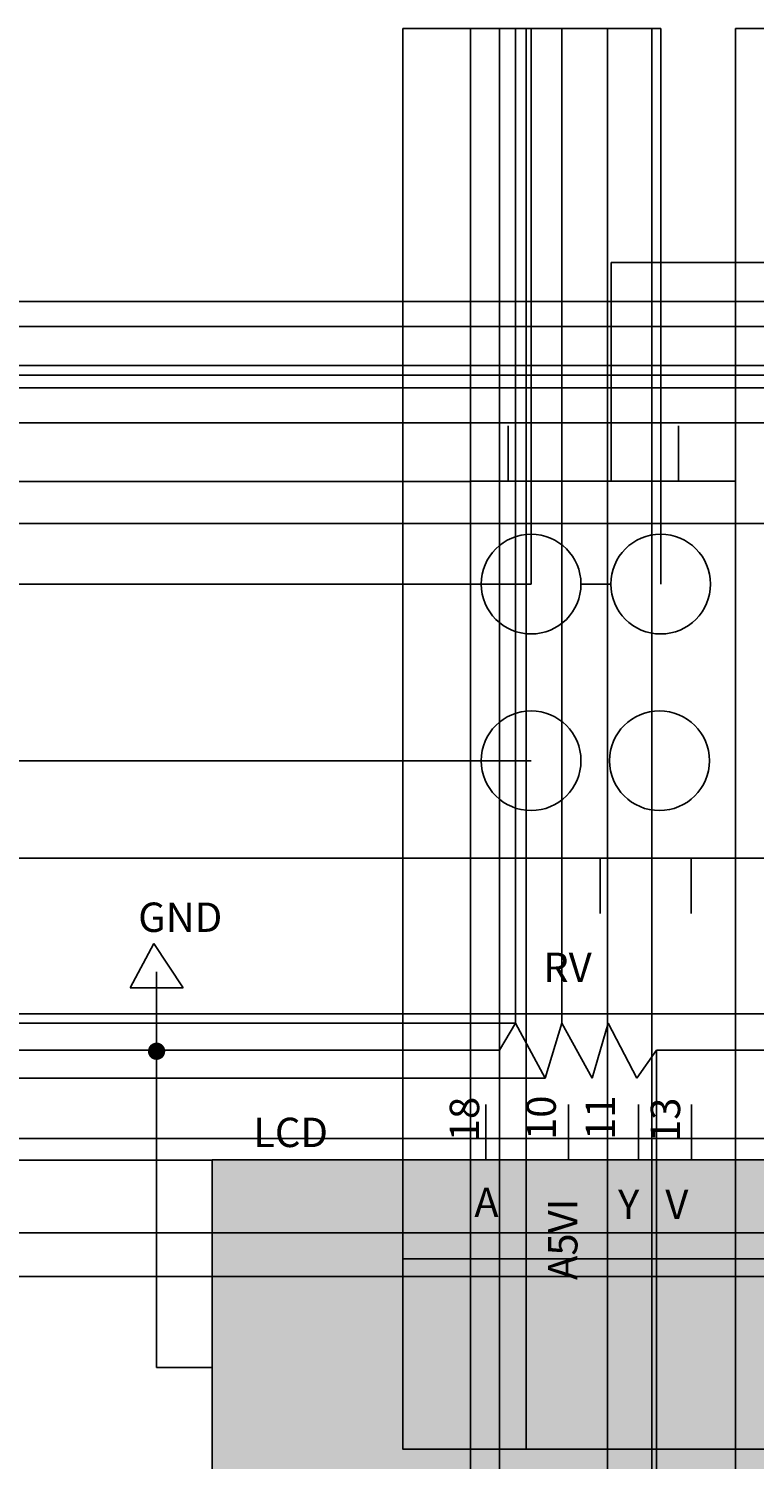
# Model space of a CAD drawing. Units: inches. Extents: x 35362 to 73946, y 43607 to 67532.
# Tile 130 of 134: x 46600 to 52056, y 56772 to 67532. Entities that reach past the tile are written whole.
import ezdxf

# ---------------------------------------------------------------- set-up
doc = ezdxf.new("R2010")
doc.units = ezdxf.units.IN
doc.header["$MEASUREMENT"] = 0
for name, color, linetype, lineweight in [('A-ANNO-DIMS', 2, 'Continuous', 18), ('E-ANNO-TEXT', 5, 'Continuous', 18), ('E-SYMB', 1, 'Continuous', 25), ('E-SYMB-PATT', 1, 'Continuous', 13), ('E-WIRE', 3, 'Continuous', 25)]:
    doc.layers.add(name, color=color, linetype=linetype, lineweight=lineweight)
doc.styles.get("Standard").update_dxf_attribs({"font": 'arial.ttf'})
doc.dimstyles.get("Standard").update_dxf_attribs({"dimtxt": 0.18, "dimasz": 0.18, "dimexe": 0.18, "dimexo": 0.0625, "dimgap": 0.09, "dimtad": 0, "dimtih": 1, "dimtoh": 1, "dimdec": 4, "dimzin": 0, "dimdsep": 46, "dimtxsty": 'Standard', "dimcen": 0.09, "dimadec": 0, "dimazin": 0, "dimtfac": 1, "dimtdec": 4, "dimtofl": 0, "dimtmove": 0, "dimatfit": 3, "dimfxl": 1, "dimtolj": 1, "dimtzin": 0, "dimarcsym": 0})

# ---------------------------------------------------------------- blocks, each defined once
blk = doc.blocks.new('*D12')
at = {"layer": 'A-ANNO-DIMS', "color": 0, "lineweight": -2, "transparency": 16777216}
for p, q in [((47979, 59023), (35362, 59023)), ((35362, 59023), (35362, 57526)), ((35362, 56029), (35362, 57526)), ((47979, 56029), (35362, 56029))]:
    blk.add_line(p, q, dxfattribs=at)
at = {"layer": 'A-ANNO-DIMS', "color": 0, "transparency": 16777216}
for points in [[(35362, 59023), (35362, 59023), (35362, 59023)], [(35362, 56029), (35362, 56029), (35362, 56029)]]:
    blk.add_solid(points, dxfattribs=at)
at = {"layer": 'Defpoints', "color": 0, "transparency": 16777216}
for p in [(47979, 59023), (35362, 56029), (47979, 56029)]:
    blk.add_point(p, dxfattribs=at)
at = {"layer": 'A-ANNO-DIMS', "color": 0, "transparency": 16777216, "insert": (35362, 57526), "char_height": 0.18, "attachment_point": 5}
blk.add_mtext('\\A1;2994.4', dxfattribs=at)
blk = doc.blocks.new('*D17')
at = {"layer": 'A-ANNO-DIMS', "color": 0, "lineweight": -2, "transparency": 16777216}
for p, q in [((49923, 61293), (49923, 43607)), ((51914, 61293), (51914, 43607)), ((49923, 43607), (50918, 43607)), ((51914, 43607), (50919, 43607))]:
    blk.add_line(p, q, dxfattribs=at)
at = {"layer": 'A-ANNO-DIMS', "color": 0, "transparency": 16777216}
for points in [[(49923, 43607), (49923, 43607), (49923, 43607)], [(51914, 43607), (51914, 43607), (51914, 43607)]]:
    blk.add_solid(points, dxfattribs=at)
at = {"layer": 'Defpoints', "color": 0, "transparency": 16777216}
for p in [(49923, 61293), (51914, 61293), (51914, 43607)]:
    blk.add_point(p, dxfattribs=at)
at = {"layer": 'A-ANNO-DIMS', "color": 0, "transparency": 16777216, "insert": (50919, 43607), "char_height": 0.18, "attachment_point": 5}
blk.add_mtext('\\A1;1990.6', dxfattribs=at)
blk = doc.blocks.new('*D18')
at = {"layer": 'A-ANNO-DIMS', "color": 0, "lineweight": -2, "transparency": 16777216}
for p, q in [((49923, 64127), (35362, 64127)), ((35362, 64127), (35362, 62711)), ((35362, 61293), (35362, 62710)), ((49923, 61293), (35362, 61293))]:
    blk.add_line(p, q, dxfattribs=at)
at = {"layer": 'A-ANNO-DIMS', "color": 0, "transparency": 16777216}
for points in [[(35362, 64127), (35362, 64127), (35362, 64127)], [(35362, 61293), (35362, 61293), (35362, 61293)]]:
    blk.add_solid(points, dxfattribs=at)
at = {"layer": 'Defpoints', "color": 0, "transparency": 16777216}
for p in [(49923, 64127), (35362, 61293), (49923, 61293)]:
    blk.add_point(p, dxfattribs=at)
at = {"layer": 'A-ANNO-DIMS', "color": 0, "transparency": 16777216, "insert": (35362, 62710), "char_height": 0.18, "attachment_point": 5}
blk.add_mtext('\\A1;2834', dxfattribs=at)
blk = doc.blocks.new('*D19')
at = {"layer": 'A-ANNO-DIMS', "color": 0, "lineweight": -2, "transparency": 16777216}
for p, q in [((50752, 63354), (50977, 63354)), ((51352, 63354), (51352, 63354)), ((51352, 63354), (51352, 63354))]:
    blk.add_line(p, q, dxfattribs=at)
at = {"layer": 'A-ANNO-DIMS', "color": 0, "transparency": 16777216}
blk.add_solid([(50977, 63354), (50977, 63354), (50977, 63354)], dxfattribs=at)
at = {"layer": 'Defpoints', "color": 0, "transparency": 16777216}
for p in [(50977, 63354), (51727, 63354)]:
    blk.add_point(p, dxfattribs=at)
at = {"layer": 'A-ANNO-DIMS', "color": 0, "transparency": 16777216, "insert": (50751, 63354), "char_height": 0.18, "attachment_point": 5}
blk.add_mtext('\\A1;8X ∅750.3', dxfattribs=at)
blk = doc.blocks.new('*D28')
at = {"layer": 'A-ANNO-DIMS', "color": 0, "lineweight": -2, "transparency": 16777216}
for p, q in [((49923, 61293), (35362, 61293)), ((35362, 61293), (35362, 60158)), ((35362, 59023), (35362, 60158)), ((47979, 59023), (35362, 59023))]:
    blk.add_line(p, q, dxfattribs=at)
at = {"layer": 'A-ANNO-DIMS', "color": 0, "transparency": 16777216}
for points in [[(35362, 61293), (35362, 61293), (35362, 61293)], [(35362, 59023), (35362, 59023), (35362, 59023)]]:
    blk.add_solid(points, dxfattribs=at)
at = {"layer": 'Defpoints', "color": 0, "transparency": 16777216}
for p in [(49923, 61293), (35362, 59023), (47979, 59023)]:
    blk.add_point(p, dxfattribs=at)
at = {"layer": 'A-ANNO-DIMS', "color": 0, "transparency": 16777216, "insert": (35362, 60158), "char_height": 0.18, "attachment_point": 5}
blk.add_mtext('\\A1;2270.0', dxfattribs=at)
blk = doc.blocks.new('*D29')
at = {"layer": 'A-ANNO-DIMS', "color": 0, "lineweight": -2, "transparency": 16777216}
for p, q in [((51914, 64128), (51914, 67532)), ((51914, 67532), (52215, 67532)), ((52518, 67532), (52216, 67532)), ((52518, 64829), (52518, 67532))]:
    blk.add_line(p, q, dxfattribs=at)
at = {"layer": 'A-ANNO-DIMS', "color": 0, "transparency": 16777216}
for points in [[(51914, 67532), (51914, 67531), (51914, 67532)], [(52518, 67532), (52518, 67531), (52518, 67532)]]:
    blk.add_solid(points, dxfattribs=at)
at = {"layer": 'Defpoints', "color": 0, "transparency": 16777216}
for p in [(52518, 67532), (52518, 64829), (51914, 64127)]:
    blk.add_point(p, dxfattribs=at)
at = {"layer": 'A-ANNO-DIMS', "color": 0, "transparency": 16777216, "insert": (52216, 67532), "char_height": 0.18, "attachment_point": 5}
blk.add_mtext('\\A1;603.9', dxfattribs=at)
blk = doc.blocks.new('*D34')
at = {"layer": 'A-ANNO-DIMS', "color": 0, "lineweight": -2, "transparency": 16777216}
for p, q in [((65336, 61293), (35362, 61293)), ((35362, 61293), (35362, 60239)), ((35362, 59185), (35362, 60239)), ((61241, 59185), (35362, 59185))]:
    blk.add_line(p, q, dxfattribs=at)
at = {"layer": 'A-ANNO-DIMS', "color": 0, "transparency": 16777216}
for points in [[(35362, 61293), (35362, 61293), (35362, 61293)], [(35362, 59185), (35362, 59185), (35362, 59185)]]:
    blk.add_solid(points, dxfattribs=at)
at = {"layer": 'Defpoints', "color": 0, "transparency": 16777216}
for p in [(65336, 61293), (35362, 59185), (61241, 59185)]:
    blk.add_point(p, dxfattribs=at)
at = {"layer": 'A-ANNO-DIMS', "color": 0, "transparency": 16777216, "insert": (35362, 60239), "char_height": 0.18, "attachment_point": 5}
blk.add_mtext('\\A1;2108.1', dxfattribs=at)
blk = doc.blocks.new('*D36')
at = {"layer": 'A-ANNO-DIMS', "color": 0, "lineweight": -2, "transparency": 16777216}
for p, q in [((68321, 60122), (35362, 60122)), ((35362, 60122), (35362, 57248)), ((35362, 54373), (35362, 57247)), ((68321, 54373), (35362, 54373))]:
    blk.add_line(p, q, dxfattribs=at)
at = {"layer": 'A-ANNO-DIMS', "color": 0, "transparency": 16777216}
for points in [[(35362, 60122), (35362, 60122), (35362, 60122)], [(35362, 54373), (35362, 54373), (35362, 54373)]]:
    blk.add_solid(points, dxfattribs=at)
at = {"layer": 'Defpoints', "color": 0, "transparency": 16777216}
for p in [(68321, 60122), (35362, 54373), (68321, 54373)]:
    blk.add_point(p, dxfattribs=at)
at = {"layer": 'A-ANNO-DIMS', "color": 0, "transparency": 16777216, "insert": (35362, 57248), "char_height": 0.18, "attachment_point": 5}
blk.add_mtext('\\A1;5749.4', dxfattribs=at)
blk = doc.blocks.new('*D45')
at = {"layer": 'A-ANNO-DIMS', "color": 0, "lineweight": -2, "transparency": 16777216}
for p, q in [((52518, 65479), (35362, 65479)), ((35362, 65479), (35362, 65154)), ((35362, 64829), (35362, 65154)), ((52518, 64829), (35362, 64829))]:
    blk.add_line(p, q, dxfattribs=at)
at = {"layer": 'A-ANNO-DIMS', "color": 0, "transparency": 16777216}
for points in [[(35362, 65479), (35362, 65479), (35362, 65479)], [(35362, 64829), (35362, 64829), (35362, 64829)]]:
    blk.add_solid(points, dxfattribs=at)
at = {"layer": 'Defpoints', "color": 0, "transparency": 16777216}
for p in [(52518, 65479), (35362, 64829), (52518, 64829)]:
    blk.add_point(p, dxfattribs=at)
at = {"layer": 'A-ANNO-DIMS', "color": 0, "transparency": 16777216, "insert": (35362, 65154), "char_height": 0.18, "attachment_point": 5}
blk.add_mtext('\\A1;650.3', dxfattribs=at)
blk = doc.blocks.new('*D46')
at = {"layer": 'A-ANNO-DIMS', "color": 0, "lineweight": -2, "transparency": 16777216}
for p, q in [((49414, 58280), (49414, 67532)), ((49414, 67532), (49876, 67532)), ((50339, 67532), (49877, 67532)), ((50340, 58280), (50340, 67532))]:
    blk.add_line(p, q, dxfattribs=at)
at = {"layer": 'A-ANNO-DIMS', "color": 0, "transparency": 16777216}
for points in [[(49414, 67532), (49414, 67531), (49414, 67532)], [(50339, 67532), (50339, 67531), (50340, 67532)]]:
    blk.add_solid(points, dxfattribs=at)
at = {"layer": 'Defpoints', "color": 0, "transparency": 16777216}
for p in [(50340, 67532), (49414, 58280), (50340, 58280)]:
    blk.add_point(p, dxfattribs=at)
at = {"layer": 'A-ANNO-DIMS', "color": 0, "transparency": 16777216, "insert": (49877, 67532), "char_height": 0.18, "attachment_point": 5}
blk.add_mtext('\\A1;925.3', dxfattribs=at)
blk = doc.blocks.new('*D47')
at = {"layer": 'A-ANNO-DIMS', "color": 0, "lineweight": -2, "transparency": 16777216}
for p, q in [((50340, 58280), (73946, 58280)), ((73946, 58280), (73946, 57564)), ((73946, 56848), (73946, 57564)), ((50340, 56848), (73946, 56848))]:
    blk.add_line(p, q, dxfattribs=at)
at = {"layer": 'A-ANNO-DIMS', "color": 0, "transparency": 16777216}
for points in [[(73946, 58280), (73946, 58280), (73946, 58280)], [(73946, 56848), (73946, 56848), (73946, 56848)]]:
    blk.add_solid(points, dxfattribs=at)
at = {"layer": 'Defpoints', "color": 0, "transparency": 16777216}
for p in [(50340, 58280), (50340, 56848), (73946, 56848)]:
    blk.add_point(p, dxfattribs=at)
at = {"layer": 'A-ANNO-DIMS', "color": 0, "transparency": 16777216, "insert": (73946, 57564), "char_height": 0.18, "attachment_point": 5}
blk.add_mtext('\\A1;1432.0', dxfattribs=at)
blk = doc.blocks.new('*D48')
at = {"layer": 'A-ANNO-DIMS', "color": 0, "lineweight": -2, "transparency": 16777216}
for p, q in [((56457, 58475), (35362, 58475)), ((35362, 58475), (35362, 58311)), ((35362, 58147), (35362, 58311)), ((56457, 58147), (35362, 58147))]:
    blk.add_line(p, q, dxfattribs=at)
at = {"layer": 'A-ANNO-DIMS', "color": 0, "transparency": 16777216}
for points in [[(35362, 58475), (35362, 58475), (35362, 58475)], [(35362, 58147), (35362, 58147), (35362, 58147)]]:
    blk.add_solid(points, dxfattribs=at)
at = {"layer": 'Defpoints', "color": 0, "transparency": 16777216}
for p in [(56457, 58475), (35362, 58147), (56457, 58147)]:
    blk.add_point(p, dxfattribs=at)
at = {"layer": 'A-ANNO-DIMS', "color": 0, "transparency": 16777216, "insert": (35362, 58311), "char_height": 0.18, "attachment_point": 5}
blk.add_mtext('\\A1;327.9', dxfattribs=at)
blk = doc.blocks.new('*D59')
at = {"layer": 'A-ANNO-DIMS', "color": 0, "lineweight": -2, "transparency": 16777216}
for p, q in [((50752, 63354), (50977, 63354)), ((51352, 63354), (51352, 63354)), ((51352, 63354), (51352, 63354))]:
    blk.add_line(p, q, dxfattribs=at)
at = {"layer": 'A-ANNO-DIMS', "color": 0, "transparency": 16777216}
blk.add_solid([(50977, 63354), (50977, 63354), (50977, 63354)], dxfattribs=at)
at = {"layer": 'Defpoints', "color": 0, "transparency": 16777216}
for p in [(50977, 63354), (51727, 63354)]:
    blk.add_point(p, dxfattribs=at)
at = {"layer": 'A-ANNO-DIMS', "color": 0, "transparency": 16777216, "insert": (50751, 63354), "char_height": 0.18, "attachment_point": 5}
blk.add_mtext('\\A1;8X ∅750.3', dxfattribs=at)
blk = doc.blocks.new('*D73')
at = {"layer": 'A-ANNO-DIMS', "color": 0, "lineweight": -2, "transparency": 16777216}
for p, q in [((59469, 64568), (35362, 64568)), ((35362, 64568), (35362, 64190)), ((35362, 63812), (35362, 64189)), ((59469, 63811), (35362, 63811))]:
    blk.add_line(p, q, dxfattribs=at)
at = {"layer": 'A-ANNO-DIMS', "color": 0, "transparency": 16777216}
for points in [[(35362, 64568), (35362, 64568), (35362, 64568)], [(35362, 63812), (35362, 63812), (35362, 63811)]]:
    blk.add_solid(points, dxfattribs=at)
at = {"layer": 'Defpoints', "color": 0, "transparency": 16777216}
for p in [(35362, 64568), (59469, 64568), (59469, 63811)]:
    blk.add_point(p, dxfattribs=at)
at = {"layer": 'A-ANNO-DIMS', "color": 0, "transparency": 16777216, "insert": (35362, 64190), "char_height": 0.18, "attachment_point": 5}
blk.add_mtext('\\A1;756.6', dxfattribs=at)
blk = doc.blocks.new('*D85')
at = {"layer": 'A-ANNO-DIMS', "color": 0, "lineweight": -2, "transparency": 16777216}
for p, q in [((50953, 49098), (50953, 67532)), ((50953, 67532), (51119, 67532)), ((51285, 67532), (51120, 67532)), ((51286, 49320), (51286, 67532))]:
    blk.add_line(p, q, dxfattribs=at)
at = {"layer": 'A-ANNO-DIMS', "color": 0, "transparency": 16777216}
for points in [[(50953, 67532), (50953, 67531), (50953, 67532)], [(51285, 67532), (51285, 67531), (51286, 67532)]]:
    blk.add_solid(points, dxfattribs=at)
at = {"layer": 'Defpoints', "color": 0, "transparency": 16777216}
for p in [(51286, 67532), (51286, 49320), (50953, 49098)]:
    blk.add_point(p, dxfattribs=at)
at = {"layer": 'A-ANNO-DIMS', "color": 0, "transparency": 16777216, "insert": (51119, 67532), "char_height": 0.18, "attachment_point": 5}
blk.add_mtext('\\A1;332.9', dxfattribs=at)
blk = doc.blocks.new('*D92')
at = {"layer": 'A-ANNO-DIMS', "color": 0, "lineweight": -2, "transparency": 16777216}
for p, q in [((50378, 63354), (50378, 67532)), ((50378, 67532), (50864, 67532)), ((51352, 67532), (50865, 67532)), ((51352, 63354), (51352, 67532))]:
    blk.add_line(p, q, dxfattribs=at)
at = {"layer": 'A-ANNO-DIMS', "color": 0, "transparency": 16777216}
for points in [[(50378, 67532), (50378, 67531), (50378, 67532)], [(51352, 67532), (51352, 67531), (51352, 67532)]]:
    blk.add_solid(points, dxfattribs=at)
at = {"layer": 'Defpoints', "color": 0, "transparency": 16777216}
for p in [(51352, 67532), (50378, 63354), (51352, 63354)]:
    blk.add_point(p, dxfattribs=at)
at = {"layer": 'A-ANNO-DIMS', "color": 0, "transparency": 16777216, "insert": (50865, 67532), "char_height": 0.18, "attachment_point": 5}
blk.add_mtext('\\A1;974.2', dxfattribs=at)
blk = doc.blocks.new('*D93')
at = {"layer": 'A-ANNO-DIMS', "color": 0, "lineweight": -2, "transparency": 16777216}
for p, q in [((50378, 63354), (35362, 63354)), ((35362, 63354), (35362, 62690)), ((35362, 62026), (35362, 62690)), ((50378, 62026), (35362, 62026))]:
    blk.add_line(p, q, dxfattribs=at)
at = {"layer": 'A-ANNO-DIMS', "color": 0, "transparency": 16777216}
for points in [[(35362, 63354), (35362, 63354), (35362, 63354)], [(35362, 62026), (35362, 62026), (35362, 62026)]]:
    blk.add_solid(points, dxfattribs=at)
at = {"layer": 'Defpoints', "color": 0, "transparency": 16777216}
for p in [(50378, 63354), (35362, 62026), (50378, 62026)]:
    blk.add_point(p, dxfattribs=at)
at = {"layer": 'A-ANNO-DIMS', "color": 0, "transparency": 16777216, "insert": (35362, 62690), "char_height": 0.18, "attachment_point": 5}
blk.add_mtext('\\A1;1328.2', dxfattribs=at)
blk = doc.blocks.new('*D94')
at = {"layer": 'A-ANNO-DIMS', "color": 0, "lineweight": -2, "transparency": 16777216}
for p, q in [((49923, 64128), (49923, 67532)), ((49923, 67532), (50150, 67532)), ((50378, 67532), (50151, 67532)), ((50378, 63354), (50378, 67532))]:
    blk.add_line(p, q, dxfattribs=at)
at = {"layer": 'A-ANNO-DIMS', "color": 0, "transparency": 16777216}
for points in [[(49923, 67532), (49923, 67531), (49923, 67532)], [(50378, 67532), (50378, 67531), (50378, 67532)]]:
    blk.add_solid(points, dxfattribs=at)
at = {"layer": 'Defpoints', "color": 0, "transparency": 16777216}
for p in [(50378, 67532), (49923, 64127), (50378, 63354)]:
    blk.add_point(p, dxfattribs=at)
at = {"layer": 'A-ANNO-DIMS', "color": 0, "transparency": 16777216, "insert": (50151, 67532), "char_height": 0.18, "attachment_point": 5}
blk.add_mtext('\\A1;454.45', dxfattribs=at)
blk = doc.blocks.new('*D95')
at = {"layer": 'A-ANNO-DIMS', "color": 0, "lineweight": -2, "transparency": 16777216}
for p, q in [((49923, 64127), (35362, 64127)), ((35362, 64127), (35362, 63741)), ((35362, 63354), (35362, 63741)), ((50378, 63354), (35362, 63354))]:
    blk.add_line(p, q, dxfattribs=at)
at = {"layer": 'A-ANNO-DIMS', "color": 0, "transparency": 16777216}
for points in [[(35362, 64127), (35362, 64127), (35362, 64127)], [(35362, 63354), (35362, 63354), (35362, 63354)]]:
    blk.add_solid(points, dxfattribs=at)
at = {"layer": 'Defpoints', "color": 0, "transparency": 16777216}
for p in [(49923, 64127), (35362, 63354), (50378, 63354)]:
    blk.add_point(p, dxfattribs=at)
at = {"layer": 'A-ANNO-DIMS', "color": 0, "transparency": 16777216, "insert": (35362, 63741), "char_height": 0.18, "attachment_point": 5}
blk.add_mtext('\\A1;773.3', dxfattribs=at)
blk = doc.blocks.new('*D98')
at = {"layer": 'A-ANNO-DIMS', "color": 0, "lineweight": -2, "transparency": 16777216}
for p, q in [((53367, 64998), (35362, 64998)), ((35362, 64998), (35362, 64913)), ((35362, 64829), (35362, 64913)), ((52518, 64829), (35362, 64829))]:
    blk.add_line(p, q, dxfattribs=at)
at = {"layer": 'A-ANNO-DIMS', "color": 0, "transparency": 16777216}
for points in [[(35362, 64998), (35362, 64998), (35362, 64998)], [(35362, 64829), (35362, 64829), (35362, 64829)]]:
    blk.add_solid(points, dxfattribs=at)
at = {"layer": 'Defpoints', "color": 0, "transparency": 16777216}
for p in [(53367, 64998), (35362, 64829), (52518, 64829)]:
    blk.add_point(p, dxfattribs=at)
at = {"layer": 'A-ANNO-DIMS', "color": 0, "transparency": 16777216, "insert": (35362, 64913), "char_height": 0.18, "attachment_point": 5}
blk.add_mtext('\\A1;169.13', dxfattribs=at)
blk = doc.blocks.new('*D101')
at = {"layer": 'A-ANNO-DIMS', "color": 0, "lineweight": -2, "transparency": 16777216}
for p, q in [((52897, 65292), (35362, 65292)), ((35362, 65291), (35362, 65109)), ((35362, 64926), (35362, 65109)), ((53151, 64926), (35362, 64926))]:
    blk.add_line(p, q, dxfattribs=at)
at = {"layer": 'A-ANNO-DIMS', "color": 0, "transparency": 16777216}
for points in [[(35362, 65291), (35362, 65291), (35362, 65292)], [(35362, 64926), (35362, 64926), (35362, 64926)]]:
    blk.add_solid(points, dxfattribs=at)
at = {"layer": 'Defpoints', "color": 0, "transparency": 16777216}
for p in [(52897, 65292), (35362, 64926), (53151, 64926)]:
    blk.add_point(p, dxfattribs=at)
at = {"layer": 'A-ANNO-DIMS', "color": 0, "transparency": 16777216, "insert": (35362, 65109), "char_height": 0.18, "attachment_point": 5}
blk.add_mtext('\\A1;365.45', dxfattribs=at)
blk = doc.blocks.new('*D107')
at = {"layer": 'A-ANNO-DIMS', "color": 0, "lineweight": -2, "transparency": 16777216}
for p, q in [((50140, 59850), (50140, 43607)), ((51321, 59850), (51321, 43607)), ((50140, 43607), (50730, 43607)), ((51321, 43607), (50731, 43607))]:
    blk.add_line(p, q, dxfattribs=at)
at = {"layer": 'A-ANNO-DIMS', "color": 0, "transparency": 16777216}
for points in [[(50140, 43607), (50140, 43607), (50140, 43607)], [(51321, 43607), (51321, 43607), (51321, 43607)]]:
    blk.add_solid(points, dxfattribs=at)
at = {"layer": 'Defpoints', "color": 0, "transparency": 16777216}
for p in [(50140, 59850), (51321, 59850), (51321, 43607)]:
    blk.add_point(p, dxfattribs=at)
at = {"layer": 'A-ANNO-DIMS', "color": 0, "transparency": 16777216, "insert": (50730, 43607), "char_height": 0.18, "attachment_point": 5}
blk.add_mtext('\\A1;1181.3', dxfattribs=at)
blk = doc.blocks.new('*D108')
at = {"layer": 'A-ANNO-DIMS', "color": 0, "lineweight": -2, "transparency": 16777216}
for p, q in [((50260, 60052), (35362, 60052)), ((35362, 60051), (35362, 59845)), ((35362, 59638), (35362, 59845)), ((50483, 59638), (35362, 59638))]:
    blk.add_line(p, q, dxfattribs=at)
at = {"layer": 'A-ANNO-DIMS', "color": 0, "transparency": 16777216}
for points in [[(35362, 60051), (35362, 60051), (35362, 60052)], [(35362, 59638), (35362, 59638), (35362, 59638)]]:
    blk.add_solid(points, dxfattribs=at)
at = {"layer": 'Defpoints', "color": 0, "transparency": 16777216}
for p in [(50260, 60052), (35362, 59638), (50483, 59638)]:
    blk.add_point(p, dxfattribs=at)
at = {"layer": 'A-ANNO-DIMS', "color": 0, "transparency": 16777216, "insert": (35362, 59845), "char_height": 0.18, "attachment_point": 5}
blk.add_mtext('\\A1;413.5', dxfattribs=at)
blk = doc.blocks.new('*D109')
at = {"layer": 'A-ANNO-DIMS', "color": 0, "lineweight": -2, "transparency": 16777216}
for p, q in [((50260, 60052), (50260, 67532)), ((50260, 67532), (50434, 67532)), ((50610, 67532), (50435, 67532)), ((50610, 60052), (50610, 67532))]:
    blk.add_line(p, q, dxfattribs=at)
at = {"layer": 'A-ANNO-DIMS', "color": 0, "transparency": 16777216}
for points in [[(50260, 67532), (50260, 67531), (50260, 67532)], [(50610, 67532), (50610, 67531), (50610, 67532)]]:
    blk.add_solid(points, dxfattribs=at)
at = {"layer": 'Defpoints', "color": 0, "transparency": 16777216}
for p in [(50610, 67532), (50260, 60052), (50610, 60052)]:
    blk.add_point(p, dxfattribs=at)
at = {"layer": 'A-ANNO-DIMS', "color": 0, "transparency": 16777216, "insert": (50435, 67532), "char_height": 0.18, "attachment_point": 5}
blk.add_mtext('\\A1;350.2', dxfattribs=at)
blk = doc.blocks.new('*D110')
at = {"layer": 'A-ANNO-DIMS', "color": 0, "lineweight": -2, "transparency": 16777216}
for p, q in [((49923, 61293), (35362, 61293)), ((35362, 61293), (35362, 60572)), ((35362, 59850), (35362, 60571)), ((50140, 59850), (35362, 59850))]:
    blk.add_line(p, q, dxfattribs=at)
at = {"layer": 'A-ANNO-DIMS', "color": 0, "transparency": 16777216}
for points in [[(35362, 61293), (35362, 61293), (35362, 61293)], [(35362, 59850), (35362, 59850), (35362, 59850)]]:
    blk.add_solid(points, dxfattribs=at)
at = {"layer": 'Defpoints', "color": 0, "transparency": 16777216}
for p in [(49923, 61293), (35362, 59850), (50140, 59850)]:
    blk.add_point(p, dxfattribs=at)
at = {"layer": 'A-ANNO-DIMS', "color": 0, "transparency": 16777216, "insert": (35362, 60572), "char_height": 0.18, "attachment_point": 5}
blk.add_mtext('\\A1;1443.2', dxfattribs=at)
blk = doc.blocks.new('*D111')
at = {"layer": 'A-ANNO-DIMS', "color": 0, "lineweight": -2, "transparency": 16777216}
for p, q in [((49923, 61293), (49923, 67532)), ((49923, 67532), (50031, 67532)), ((50139, 67532), (50032, 67532)), ((50140, 59850), (50140, 67532))]:
    blk.add_line(p, q, dxfattribs=at)
at = {"layer": 'A-ANNO-DIMS', "color": 0, "transparency": 16777216}
for points in [[(49923, 67532), (49923, 67531), (49923, 67532)], [(50139, 67532), (50139, 67531), (50140, 67532)]]:
    blk.add_solid(points, dxfattribs=at)
at = {"layer": 'Defpoints', "color": 0, "transparency": 16777216}
for p in [(50140, 67532), (49923, 61293), (50140, 59850)]:
    blk.add_point(p, dxfattribs=at)
at = {"layer": 'A-ANNO-DIMS', "color": 0, "transparency": 16777216, "insert": (50031, 67532), "char_height": 0.18, "attachment_point": 5}
blk.add_mtext('\\A1;216.26', dxfattribs=at)
blk = doc.blocks.new('*D118')
at = {"layer": 'A-ANNO-DIMS', "color": 0, "lineweight": -2, "transparency": 16777216}
for p, q in [((50378, 63354), (50378, 63354)), ((50378, 63354), (50378, 63354)), ((50978, 63354), (50753, 63354))]:
    blk.add_line(p, q, dxfattribs=at)
at = {"layer": 'A-ANNO-DIMS', "color": 0, "transparency": 16777216}
blk.add_solid([(50753, 63354), (50753, 63354), (50753, 63354)], dxfattribs=at)
at = {"layer": 'Defpoints', "color": 0, "transparency": 16777216}
for p in [(50003, 63354), (50753, 63354)]:
    blk.add_point(p, dxfattribs=at)
at = {"layer": 'A-ANNO-DIMS', "color": 0, "transparency": 16777216, "insert": (50979, 63354), "char_height": 0.18, "attachment_point": 5}
blk.add_mtext('\\A1;8X ∅750.3', dxfattribs=at)

msp = doc.modelspace()

# ---------------------------------------------------------------- hatches: boundary and pattern name
at = {"layer": 'E-SYMB-PATT'}
h = msp.add_hatch(color=256, dxfattribs=at)
h.dxf.hatch_style = 1
h.paths.add_polyline_path([(47561.92, 59906.061, 0.414213562), (47496.715, 59840.856, 0.414213562), (47561.92, 59775.651)])
h.paths.add_polyline_path([(47561.92, 59906.061), (47561.92, 59775.651, 0.414213562), (47627.125, 59840.856, 0.414213562)])
h = msp.add_hatch(color=256, dxfattribs=at)
h.dxf.hatch_style = 1
h.paths.add_polyline_path([(53109.76, 56028.836), (53109.76, 59023.276), (47978.665, 59023.276), (47978.665, 56028.836)])

# ---------------------------------------------------------------- linework, layer by layer
at = {"layer": 'E-SYMB'}
for p, q in [((50978.723, 65771.512), (52897.48, 65771.512)), ((50204.468, 64543.754), (50204.468, 64127.442)), ((51485.882, 64543.754), (51485.882, 64127.442)), ((50340.575, 61293.286), (50340.575, 60876.974)), ((50898.169, 61293.286), (50898.169, 60876.974)), ((51581.922, 61293.286), (51581.922, 60876.974)), ((47540.642, 60650.854), (47362.353, 60317.921)), ((47762.353, 60317.921), (47540.642, 60650.854)), ((47562.353, 60317.921), (47362.353, 60317.921)), ((47562.353, 59850.077), (47562.353, 60317.921)), ((47562.353, 60317.921), (47762.353, 60317.921)), ((50139.563, 59850.077), (50259.724, 60051.661)), ((50259.724, 60051.661), (50483.095, 59638.132)), ((50483.095, 59638.132), (50609.914, 60051.661)), ((50609.914, 60051.661), (50836.506, 59638.132)), ((50836.506, 59638.132), (50956.669, 60051.661)), ((50956.669, 60051.661), (51172.962, 59638.132)), ((49903.185, 59850.077), (50139.563, 59850.077)), ((51172.962, 59638.132), (51320.813, 59850.077)), ((51320.813, 59850.077), (51612.51, 59850.077)), ((50038.496, 59439.589), (50038.496, 59023.276)), ((50658.098, 59439.589), (50658.098, 59023.276)), ((51185.224, 59439.589), (51185.224, 59023.276)), ((51582.878, 59439.589), (51582.878, 59023.276)), ((47978.665, 57463.179), (47562.353, 57463.179))]:
    msp.add_line(p, q, dxfattribs=at)
for points in [[(49923.307, 64127.442), (51913.931, 64127.442), (51913.931, 61293.286), (49923.307, 61293.286)], [(47978.665, 59023.276), (53109.76, 59023.276), (53109.76, 56028.836), (47978.665, 56028.836)], [(49414.26, 58279.988), (50339.524, 58279.988), (50339.524, 56847.99), (49414.26, 56847.99)]]:
    msp.add_lwpolyline(points, close=True, dxfattribs=at)
for centre in [(50377.76, 63354.176), (51351.915, 63354.176), (50377.76, 62026.025), (51342.885, 62026.025)]:
    msp.add_circle(centre, 375.127, dxfattribs=at)
at = {"layer": 'E-WIRE'}
for p, q in [((50978.723, 65771.512), (50978.723, 64127.442)), ((47562.353, 60439.178), (47562.353, 57463.179)), ((47562.353, 59850.077), (49903.185, 59850.077)), ((51612.51, 59850.077), (53526.072, 59850.077))]:
    msp.add_line(p, q, dxfattribs=at)

# ---------------------------------------------------------------- texts
at = {"layer": 'E-ANNO-TEXT'}
for s, p in [('GND', (47423.417, 60738.292)), ('RV', (50468.698, 60362.066)), ('LCD', (48287.73, 59120.329)), ('A', (49950.554, 58593.417)), ('Y', (51031.177, 58579.088)), ('V', (51386.782, 58579.088))]:
    msp.add_text(s, height=220.866, dxfattribs=at).set_placement(p)
for s, p in [('18', (49986.996, 59163.807)), ('10', (50563.845, 59173.51)), ('11', (51008.62, 59173.51)), ('13', (51498.496, 59158.048)), ('A5VI', (50726.347, 58120.572))]:
    msp.add_text(s, height=220.866, rotation=90, dxfattribs=at).set_placement(p)

# ---------------------------------------------------------------- dimensions: what is measured, and where the dimension line sits
at = {"layer": 'A-ANNO-DIMS'}
for base, p1, p2, override, picture, middle in [((50339.524, 67531.512), (49414.26, 58279.988), (50339.524, 58279.988), {"dimdec": 1, "dimlfac": 1, "dimrnd": 0, "dimzin": 0, "dimdsep": 46, "dimlunit": 2}, '*D46', (49876.892, 67531.512)), ((50377.76, 67531.512), (49923.307, 64127.442), (50377.76, 63354.176), {"dimdec": 2, "dimlfac": 1, "dimrnd": 0, "dimzin": 0, "dimdsep": 46, "dimlunit": 2}, '*D94', (50150.533, 67531.512)), ((50139.563, 67531.512), (49923.307, 61293.286), (50139.563, 59850.077), {"dimdec": 2, "dimlfac": 1, "dimrnd": 0, "dimzin": 0, "dimdsep": 46, "dimlunit": 2}, '*D111', (50031.435, 67531.512)), ((50609.914, 67531.512), (50259.724, 60051.661), (50609.914, 60051.661), {"dimdec": 1, "dimlfac": 1, "dimrnd": 0, "dimzin": 0, "dimdsep": 46, "dimlunit": 2}, '*D109', (50434.819, 67531.512)), ((51351.915, 67531.512), (50377.76, 63354.176), (51351.915, 63354.176), {"dimdec": 1, "dimlfac": 1, "dimrnd": 0, "dimzin": 0, "dimdsep": 46, "dimlunit": 2}, '*D92', (50864.837, 67531.512)), ((51285.595, 67531.512), (50952.662, 49098.368), (51285.595, 49320.079), {"dimdec": 1, "dimlfac": 1, "dimrnd": 0, "dimzin": 0, "dimdsep": 46, "dimlunit": 2}, '*D85', (51119.128, 67531.512)), ((52517.798, 67531.512), (51913.931, 64127.442), (52517.798, 64828.556), {"dimdec": 1, "dimlfac": 1, "dimrnd": 0, "dimzin": 0, "dimdsep": 46, "dimlunit": 2}, '*D29', (52215.864, 67531.512)), ((51913.931, 43606.859), (49923.307, 61293.286), (51913.931, 61293.286), {"dimdec": 1, "dimlfac": 1, "dimrnd": 0, "dimzin": 0, "dimdsep": 46, "dimlunit": 2}, '*D17', (50918.619, 43606.859)), ((51320.8133, 43606.859), (50139.5627, 59850.0769), (51320.8133, 59850.0769), {"dimdec": 1, "dimlfac": 1, "dimrnd": 0, "dimzin": 0, "dimdsep": 46, "dimlunit": 2}, '*D107', (50730.188, 43606.859))]:
    dim = msp.add_linear_dim(base=base, p1=p1, p2=p2, dimstyle='Standard', override=override, dxfattribs=at)
    dim.commit()
    dim.dimension.update_dxf_attribs({"geometry": picture, "text_midpoint": middle})
for base, p1, p2, override, picture, middle in [((35361.949, 64828.556), (52517.798, 65478.87), (52517.798, 64828.556), {"dimdec": 1, "dimlfac": 1, "dimrnd": 0, "dimzin": 0, "dimdsep": 46, "dimlunit": 2}, '*D45', (35361.949, 65153.713)), ((35361.949, 64926.138), (52897.48, 65291.589), (53150.662, 64926.138), {"dimdec": 2, "dimlfac": 1, "dimrnd": 0, "dimzin": 0, "dimdsep": 46, "dimlunit": 2}, '*D101', (35361.949, 65108.863)), ((35361.949, 64828.556), (53366.766, 64997.683), (52517.798, 64828.556), {"dimdec": 2, "dimlfac": 1, "dimrnd": 0, "dimzin": 0, "dimdsep": 46, "dimlunit": 2}, '*D98', (35361.949, 64913.119)), ((35361.949, 64567.972), (59468.796, 63811.354), (59468.796, 64567.972), {"dimdec": 1, "dimlfac": 1, "dimrnd": 0, "dimzin": 0, "dimdsep": 46, "dimlunit": 2}, '*D73', (35361.949, 64189.663)), ((35361.949, 63354.176), (49923.307, 64127.442), (50377.76, 63354.176), {"dimdec": 1, "dimlfac": 1, "dimrnd": 0, "dimzin": 0, "dimdsep": 46, "dimlunit": 2}, '*D95', (35361.949, 63740.809)), ((35361.949, 61293.286), (49923.307, 64127.442), (49923.307, 61293.286), {"dimdec": 0, "dimlfac": 1, "dimrnd": 0, "dimzin": 0, "dimdsep": 46, "dimlunit": 2}, '*D18', (35361.949, 62710.364)), ((35361.949, 62026.025), (50377.76, 63354.176), (50377.76, 62026.025), {"dimdec": 1, "dimlfac": 1, "dimrnd": 0, "dimzin": 0, "dimdsep": 46, "dimlunit": 2}, '*D93', (35361.949, 62690.1)), ((35361.949, 59023.276), (49923.307, 61293.286), (47978.665, 59023.276), {"dimdec": 1, "dimlfac": 1, "dimrnd": 0, "dimzin": 0, "dimdsep": 46, "dimlunit": 2}, '*D28', (35361.949, 60158.281)), ((35361.949, 59185.144), (65336.016, 61293.286), (61240.907, 59185.144), {"dimdec": 1, "dimlfac": 1, "dimrnd": 0, "dimzin": 0, "dimdsep": 46, "dimlunit": 2}, '*D34', (35361.949, 60239.215)), ((35361.949, 59850.077), (49923.307, 61293.286), (50139.563, 59850.077), {"dimdec": 1, "dimlfac": 1, "dimrnd": 0, "dimzin": 0, "dimdsep": 46, "dimlunit": 2}, '*D110', (35361.949, 60571.681)), ((35361.949, 54372.948), (68320.871, 60122.346), (68320.871, 54372.948), {"dimdec": 1, "dimlfac": 1, "dimrnd": 0, "dimzin": 0, "dimdsep": 46, "dimlunit": 2}, '*D36', (35361.949, 57247.647)), ((35361.949, 59638.132), (50259.724, 60051.661), (50483.095, 59638.132), {"dimdec": 1, "dimlfac": 1, "dimrnd": 0, "dimzin": 0, "dimdsep": 46, "dimlunit": 2}, '*D108', (35361.949, 59844.897)), ((35361.949, 56028.836), (47978.665, 59023.276), (47978.665, 56028.836), {"dimdec": 1, "dimlfac": 1, "dimrnd": 0, "dimzin": 0, "dimdsep": 46, "dimlunit": 2}, '*D12', (35361.949, 57526.056)), ((35361.949, 58146.959), (56457.29, 58474.868), (56457.29, 58146.959), {"dimdec": 1, "dimlfac": 1, "dimrnd": 0, "dimzin": 0, "dimdsep": 46, "dimlunit": 2}, '*D48', (35361.949, 58310.914)), ((73945.646, 56847.99), (50339.524, 58279.988), (50339.524, 56847.99), {"dimdec": 1, "dimlfac": 1, "dimrnd": 0, "dimzin": 0, "dimdsep": 46, "dimlunit": 2}, '*D47', (73945.646, 57563.989))]:
    dim = msp.add_linear_dim(base=base, p1=p1, p2=p2, angle=90, dimstyle='Standard', override=override, dxfattribs=at)
    dim.commit()
    dim.dimension.update_dxf_attribs({"geometry": picture, "text_midpoint": middle})
for p1, p2, picture, middle in [((50002.633, 63354.177), (50752.886, 63354.176), '*D118', (50977.962, 63354.176)), ((51727.041, 63354.472), (50976.788, 63353.881), '*D19', (50751.712, 63353.704)), ((51727.041, 63354.472), (50976.788, 63353.881), '*D59', (50751.712, 63353.704))]:
    dim = msp.add_diameter_dim_2p(p1=p1, p2=p2, text='8X <>', dimstyle='Standard', override={"dimdec": 1, "dimlfac": 1, "dimrnd": 0, "dimzin": 0, "dimdsep": 46, "dimlunit": 2}, dxfattribs=at)
    dim.commit()
    dim.dimension.update_dxf_attribs({"geometry": picture, "text_midpoint": middle, "dimtype": 163})

doc.saveas('drawing.dxf')
